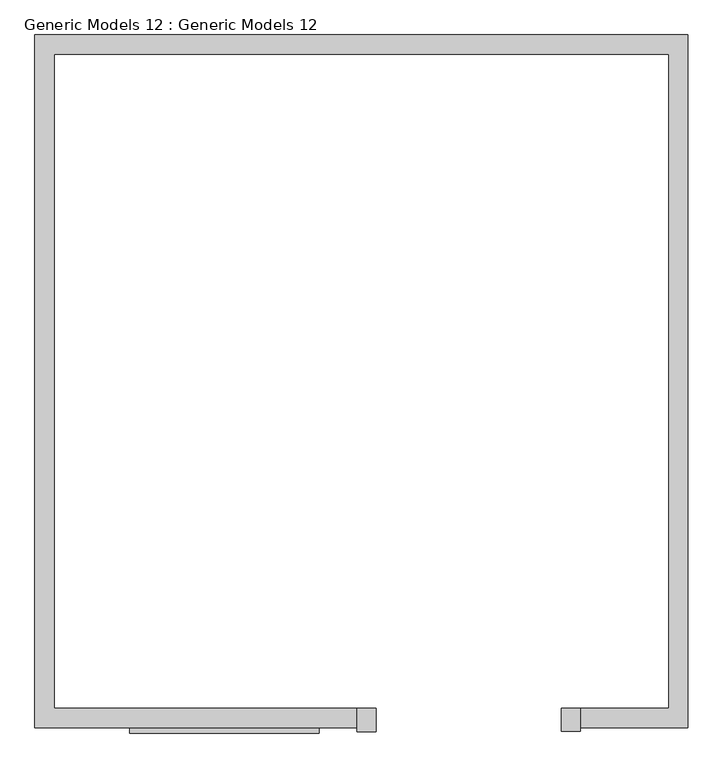
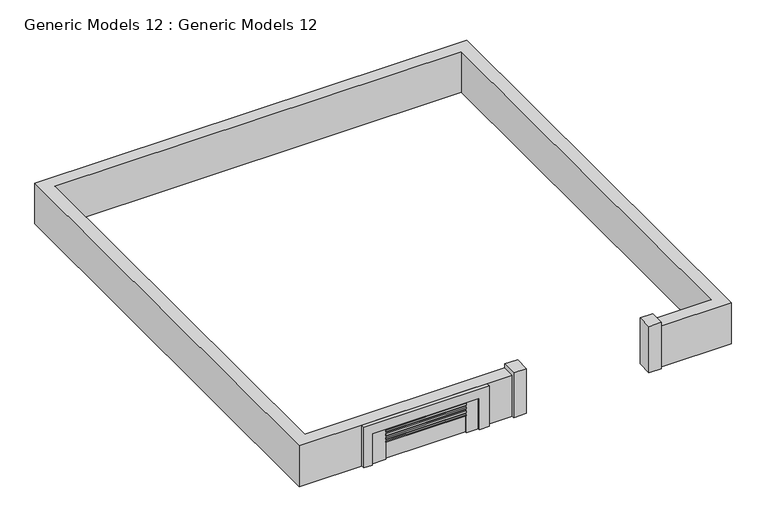
"""IFC4 building model written with IfcOpenShell, lengths in millimetres: proxy geometry, Generic Models 12 : Generic Models 12."""

from ifc_helpers import new_model, si_unit, frame, origin, place, context, project, spatial, polyline, outline, extrude, source, transform, mapped, element, save


def generic_models_12_generic_models_12_a8744921(model_context):
    return source(origin(), model_context, "Body", "SweptSolid", [
        extrude(outline(polyline([(-21722.1696364, -16496.9752569), (-13272.6784466, -16496.9752569), (-13272.6784466, -17030.3752569), (-22255.5696364, -17030.3752569), (-22255.5696364, 2275.9041488), (-4043.3695233, 2275.9041488), (-4043.3695233, -17030.3752569), (-7037.2901337, -17030.3752569), (-7037.2901337, -16496.9752569), (-4576.7695233, -16496.9752569), (-4576.7695233, 1742.5041488), (-21722.1696364, 1742.5041488), (-21722.1696364, -16496.9752569)])), frame((0.0, 0.0, -304.8), z_axis=(0.0, 0.0, 1.0), x_axis=(1.0, 0.0, 0.0)), (0.0, 0.0, 1.0), 1817.7505935),
        extrude(outline(polyline([(-15251.9881478, -17106.5752569), (-18655.4995068, -17106.5752569), (-18655.4995068, -17030.3752569), (-15251.9881478, -17030.3752569), (-15251.9881478, -17106.5752569)])), frame((0.0, 0.0, 918.154632), z_axis=(0.0, 0.0, 1.0), x_axis=(1.0, 0.0, 0.0)), (0.0, 0.0, 1.0), 75.6593747),
        extrude(outline(polyline([(-15251.9881478, -17106.5752569), (-18655.4995068, -17106.5752569), (-18655.4995068, -17030.3752569), (-15251.9881478, -17030.3752569), (-15251.9881478, -17106.5752569)])), frame((0.0, 0.0, 748.7408893), z_axis=(0.0, 0.0, 1.0), x_axis=(1.0, 0.0, 0.0)), (0.0, 0.0, 1.0), 77.8387466),
        extrude(outline(polyline([(-15251.9881478, -17106.5752569), (-18655.4995068, -17106.5752569), (-18655.4995068, -17030.3752569), (-15251.9881478, -17030.3752569), (-15251.9881478, -17106.5752569)])), frame((0.0, 0.0, 583.9058964), z_axis=(0.0, 0.0, 1.0), x_axis=(1.0, 0.0, 0.0)), (0.0, 0.0, 1.0), 77.8387466),
        extrude(outline(polyline([(-15251.9881478, -17106.5752569), (-18655.4995068, -17106.5752569), (-18655.4995068, -17030.3752569), (-15251.9881478, -17030.3752569), (-15251.9881478, -17106.5752569)])), frame((0.0, 0.0, 445.5306109), z_axis=(0.0, 0.0, 1.0), x_axis=(1.0, 0.0, 0.0)), (0.0, 0.0, 1.0), 51.3790393),
        extrude(outline(polyline([(-14748.6938869, -17106.5752569), (-15251.9881478, -17106.5752569), (-15251.9881478, -17030.3752569), (-14748.6938869, -17030.3752569), (-14748.6938869, -17106.5752569)])), frame((0.0, 0.0, -304.8), z_axis=(0.0, 0.0, 1.0), x_axis=(1.0, 0.0, 0.0)), (0.0, 0.0, 1.0), 1403.8426986),
        extrude(outline(polyline([(-18655.4995068, -17106.5752569), (-19257.3454048, -17106.5752569), (-19257.3454048, -17030.3752569), (-18655.4995068, -17030.3752569), (-18655.4995068, -17106.5752569)])), frame((0.0, 0.0, -304.8), z_axis=(0.0, 0.0, 1.0), x_axis=(1.0, 0.0, 0.0)), (0.0, 0.0, 1.0), 1403.8426986),
        extrude(outline(polyline([(1512.9505935, -19617.7171957), (-304.8, -19617.7171957), (-304.8, -19257.3454048), (1099.0426986, -19257.3454048), (1099.0426986, -14748.6938869), (-304.8, -14748.6938869), (-304.8, -14336.2607949), (1512.9505935, -14336.2607949), (1512.9505935, -19617.7171957)])), frame((0.0, -17182.7752569, 0.0), z_axis=(0.0, 1.0, 0.0), x_axis=(0.0, 0.0, 1.0)), (0.0, 0.0, 1.0), 152.4),
        extrude(outline(polyline([(-12739.2784466, -16496.9752569), (-12739.2784466, -17144.6752569), (-13272.6784466, -17144.6752569), (-13272.6784466, -16496.9752569), (-12739.2784466, -16496.9752569)])), frame((0.0, 0.0, -304.8), z_axis=(0.0, 0.0, 1.0), x_axis=(1.0, 0.0, 0.0)), (0.0, 0.0, 1.0), 1998.2983763),
        extrude(outline(polyline([(-7570.6901337, -17138.4838627), (-7570.6901337, -16496.9752569), (-7037.2901337, -16496.9752569), (-7037.2901337, -17138.4838627), (-7570.6901337, -17138.4838627)])), frame((0.0, 0.0, -304.8), z_axis=(0.0, 0.0, 1.0), x_axis=(1.0, 0.0, 0.0)), (0.0, 0.0, 1.0), 2054.6639552),
    ])


if __name__ == "__main__":
    model = new_model("IFC4")
    model_context = context("Model", 3, world=origin())
    ifc_project = project(units=[si_unit("LENGTHUNIT", "METRE", prefix="MILLI")], contexts=[model_context])
    site = spatial("IfcSite", under=ifc_project)
    building = spatial("IfcBuilding", under=site)
    placement = place(None, origin())
    generic_models_12_generic_models_12_shape = generic_models_12_generic_models_12_a8744921(model_context)
    element("IfcBuildingElementProxy", 1, Name="Generic Models 12 : Generic Models 12", ObjectType="Generic Models 12 : Generic Models 12", at=placement, inside=building, context=model_context, shape_type="MappedRepresentation", body=[
        mapped(generic_models_12_generic_models_12_shape, transform((0.0, 0.0, 0.0), x_axis=(1.0, 0.0, 0.0), y_axis=(0.0, 1.0, 0.0), z_axis=(0.0, 0.0, 1.0))),
    ])
    save(model, "model.ifc")
